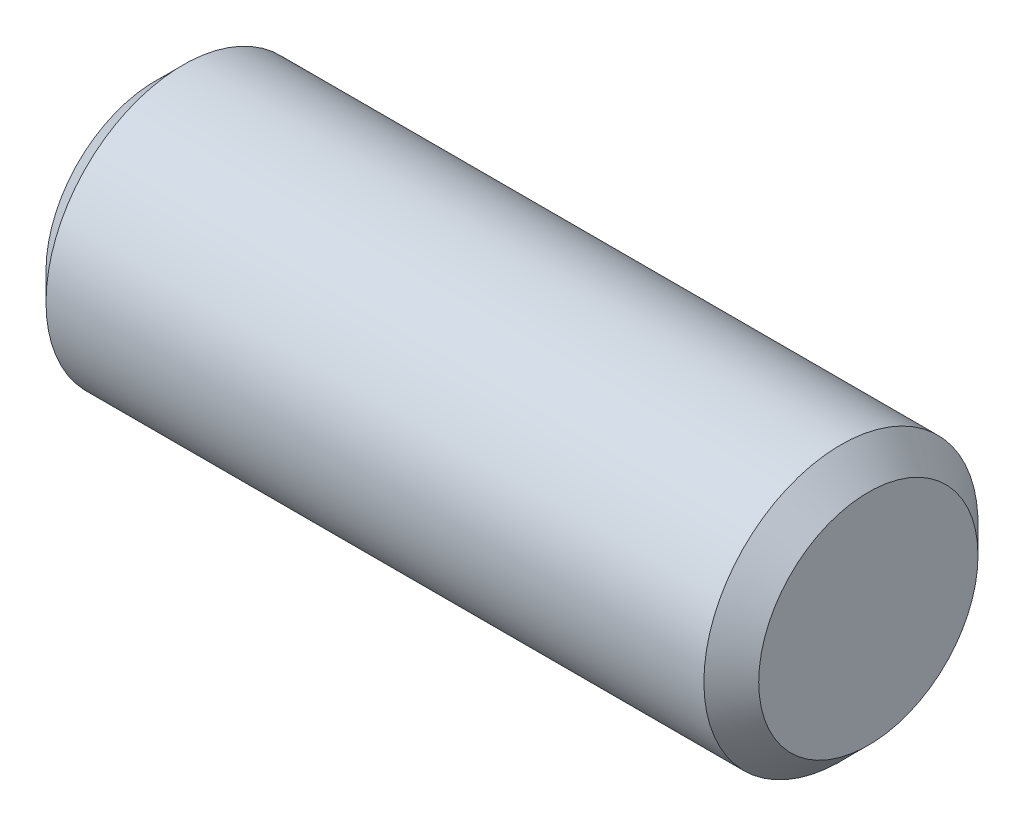
SolidWorks part; units mm, degrees
material "Plain Carbon Steel"
ref_plane "Front Plane" through (0, 0, 0) normal (0, 0, 1) x (1, 0, 0)
ref_plane "Top Plane" through (0, 0, 0) normal (0, 1, 0) x (1, 0, 0)
ref_plane "Right Plane" through (0, 0, 0) normal (1, 0, 0) x (0, 0, -1)
sketch "Pin Profile Ø20" plane through (0, 0, 0) normal (1, 0, 0) x (0, 0, -1)
  circle A0 centre (0, 0) radius 10
  dimension "D1" = 20
extrude "Pin Body Ø20x52" add sketch "Pin Profile Ø20" along normal mid plane 52
chamfer "End Chamfers 2x45°" distance 2 angle 45 2 edges at (-26, 0, -10) (26, 0, -10)
